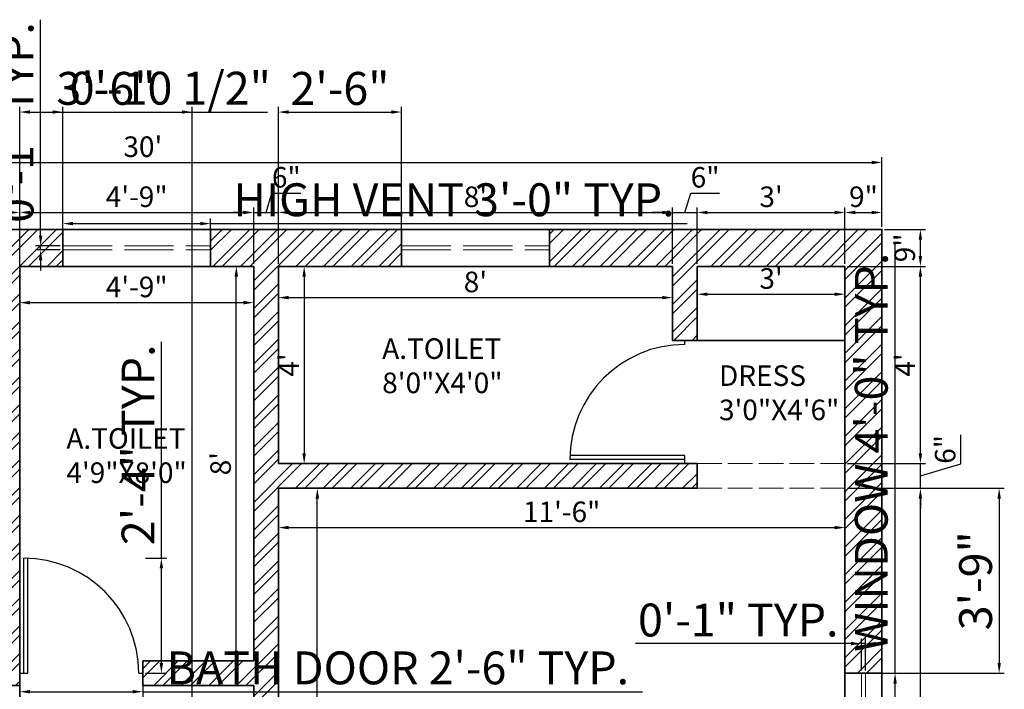
# Model space of a CAD drawing. Units: inches. Extents: x 3595 to 4516, y 2363 to 2965.
# Tile 5 of 12: x 3790 to 4030, y 2791 to 2954. Entities that reach past the tile are written whole.
import ezdxf

# ---------------------------------------------------------------- set-up
doc = ezdxf.new("R2010")
doc.units = ezdxf.units.IN
doc.linetypes.add('ACAD_ISO02W100', pattern=[15, 12, -3])
for name, color, linetype, lineweight in [('A-ANNO-DIMS', 2, 'Continuous', 18), ('A-AREA-IDEN', 7, 'Continuous', 18), ('A-DOOR', 4, 'Continuous', 25), ('A-GLAZ', 4, 'Continuous', 18), ('A-GLAZ-HIGH', 4, 'ACAD_ISO02W100', 18), ('A-WALL', 7, 'Continuous', 35), ('A-WALL-OVHD', 7, 'ACAD_ISO02W100', 18)]:
    doc.layers.add(name, color=color, linetype=linetype, lineweight=lineweight)
doc.layers.add('A-WALL-PATT', color=251, linetype='Continuous', lineweight=13, true_color=0x636466)
doc.styles.get("Standard").update_dxf_attribs({"font": 'arial.ttf'})
doc.dimstyles.new('ISO-25', dxfattribs={"dimtxt": 8, "dimasz": 2.5, "dimexe": 1.25, "dimexo": 0.625, "dimtad": 1, "dimdec": 1, "dimlunit": 3, "dimtxsty": 'Standard', "dimcen": 2.5, "dimadec": 0, "dimazin": 0, "dimtfac": 1, "dimtdec": 1, "dimtmove": 0, "dimatfit": 3, "dimfxl": 1, "dimarcsym": 0})

# ---------------------------------------------------------------- blocks, each defined once
blk = doc.blocks.new('D2')
for p, q in [((1, 0), (1, 28)), ((2, 0), (2, 27.98)), ((0, 0), (2, 0)), ((29, 0), (30, 0))]:
    blk.add_line(p, q)
at = {"ltscale": 0.5}
blk.add_arc((1, 0), 28, 0, 90, dxfattribs=at)
blk = doc.blocks.new('*D39')
at = {"layer": 'A-ANNO-DIMS', "color": 0, "lineweight": -2, "transparency": 16777216}
for p, q in [((3853.52, 2840.04), (3863.63, 2840.04)), ((3862.38, 2704.54), (3862.38, 2837.54)), ((3853.52, 2702.04), (3863.63, 2702.04))]:
    blk.add_line(p, q, dxfattribs=at)
at = {"layer": 'A-ANNO-DIMS', "color": 0, "transparency": 16777216}
for points in [[(3861.96, 2837.54), (3862.79, 2837.54), (3862.38, 2840.04)], [(3861.96, 2704.54), (3862.79, 2704.54), (3862.38, 2702.04)]]:
    blk.add_solid(points, dxfattribs=at)
at = {"layer": 'Defpoints', "color": 0, "transparency": 16777216}
for p in [(3852.89, 2840.04), (3862.38, 2840.04), (3852.89, 2702.04)]:
    blk.add_point(p, dxfattribs=at)
at = {"layer": 'A-ANNO-DIMS', "color": 0, "transparency": 16777216, "insert": (3859.2, 2771.04), "char_height": 5, "attachment_point": 5, "rotation": 90}
blk.add_mtext('11\'-6"', dxfattribs=at)
blk = doc.blocks.new('*D40')
at = {"layer": 'A-ANNO-DIMS', "color": 0, "lineweight": -2, "transparency": 16777216}
for p, q in [((3852.89, 2839.42), (3852.89, 2829.23)), ((3990.89, 2839.42), (3990.89, 2829.23)), ((3855.39, 2830.48), (3988.39, 2830.48))]:
    blk.add_line(p, q, dxfattribs=at)
at = {"layer": 'A-ANNO-DIMS', "color": 0, "transparency": 16777216}
for points in [[(3855.39, 2830.9), (3855.39, 2830.06), (3852.89, 2830.48)], [(3988.39, 2830.9), (3988.39, 2830.06), (3990.89, 2830.48)]]:
    blk.add_solid(points, dxfattribs=at)
at = {"layer": 'Defpoints', "color": 0, "transparency": 16777216}
for p in [(3852.89, 2840.04), (3990.89, 2840.04), (3990.89, 2830.48)]:
    blk.add_point(p, dxfattribs=at)
at = {"layer": 'A-ANNO-DIMS', "color": 0, "transparency": 16777216, "insert": (3921.89, 2833.66), "char_height": 5, "attachment_point": 5}
blk.add_mtext('11\'-6"', dxfattribs=at)
blk = doc.blocks.new('*D41')
at = {"layer": 'A-ANNO-DIMS', "color": 0, "lineweight": -2, "transparency": 16777216}
for p, q in [((3852.89, 2893.42), (3852.89, 2885.19)), ((3948.89, 2893.42), (3948.89, 2885.19)), ((3855.39, 2886.44), (3946.39, 2886.44))]:
    blk.add_line(p, q, dxfattribs=at)
at = {"layer": 'A-ANNO-DIMS', "color": 0, "transparency": 16777216}
for points in [[(3855.39, 2886.85), (3855.39, 2886.02), (3852.89, 2886.44)], [(3946.39, 2886.85), (3946.39, 2886.02), (3948.89, 2886.44)]]:
    blk.add_solid(points, dxfattribs=at)
at = {"layer": 'Defpoints', "color": 0, "transparency": 16777216}
for p in [(3852.89, 2894.04), (3948.89, 2894.04), (3948.89, 2886.44)]:
    blk.add_point(p, dxfattribs=at)
at = {"layer": 'A-ANNO-DIMS', "color": 0, "transparency": 16777216, "insert": (3900.89, 2889.61), "char_height": 5, "attachment_point": 5}
blk.add_mtext("8'", dxfattribs=at)
blk = doc.blocks.new('*D42')
at = {"layer": 'A-ANNO-DIMS', "color": 0, "lineweight": -2, "transparency": 16777216}
for p, q in [((3853.52, 2894.04), (3860.42, 2894.04)), ((3859.17, 2891.54), (3859.17, 2848.54)), ((3853.52, 2846.04), (3860.42, 2846.04))]:
    blk.add_line(p, q, dxfattribs=at)
at = {"layer": 'A-ANNO-DIMS', "color": 0, "transparency": 16777216}
for points in [[(3858.76, 2891.54), (3859.59, 2891.54), (3859.17, 2894.04)], [(3858.76, 2848.54), (3859.59, 2848.54), (3859.17, 2846.04)]]:
    blk.add_solid(points, dxfattribs=at)
at = {"layer": 'Defpoints', "color": 0, "transparency": 16777216}
for p in [(3852.89, 2894.04), (3852.89, 2846.04), (3859.17, 2846.04)]:
    blk.add_point(p, dxfattribs=at)
at = {"layer": 'A-ANNO-DIMS', "color": 0, "transparency": 16777216, "insert": (3856.05, 2870.04), "char_height": 5, "attachment_point": 5, "rotation": 90}
blk.add_mtext("4'", dxfattribs=at)
blk = doc.blocks.new('*D43')
at = {"layer": 'A-ANNO-DIMS', "color": 0, "lineweight": -2, "transparency": 16777216}
for p, q in [((3954.89, 2893.42), (3954.89, 2886.01)), ((3990.89, 2893.42), (3990.89, 2886.01)), ((3957.39, 2887.26), (3988.39, 2887.26))]:
    blk.add_line(p, q, dxfattribs=at)
at = {"layer": 'A-ANNO-DIMS', "color": 0, "transparency": 16777216}
for points in [[(3957.39, 2887.67), (3957.39, 2886.84), (3954.89, 2887.26)], [(3988.39, 2887.67), (3988.39, 2886.84), (3990.89, 2887.26)]]:
    blk.add_solid(points, dxfattribs=at)
at = {"layer": 'Defpoints', "color": 0, "transparency": 16777216}
for p in [(3954.89, 2894.04), (3990.89, 2894.04), (3990.89, 2887.26)]:
    blk.add_point(p, dxfattribs=at)
at = {"layer": 'A-ANNO-DIMS', "color": 0, "transparency": 16777216, "insert": (3972.89, 2890.44), "char_height": 5, "attachment_point": 5}
blk.add_mtext("3'", dxfattribs=at)
blk = doc.blocks.new('*D44')
at = {"layer": 'A-ANNO-DIMS', "color": 0, "lineweight": -2, "transparency": 16777216}
for p, q in [((3789.89, 2893.42), (3789.89, 2883.96)), ((3846.89, 2893.42), (3846.89, 2883.96)), ((3792.39, 2885.21), (3844.39, 2885.21))]:
    blk.add_line(p, q, dxfattribs=at)
at = {"layer": 'A-ANNO-DIMS', "color": 0, "transparency": 16777216}
for points in [[(3792.39, 2885.63), (3792.39, 2884.79), (3789.89, 2885.21)], [(3844.39, 2885.63), (3844.39, 2884.79), (3846.89, 2885.21)]]:
    blk.add_solid(points, dxfattribs=at)
at = {"layer": 'Defpoints', "color": 0, "transparency": 16777216}
for p in [(3789.89, 2894.04), (3846.89, 2894.04), (3846.89, 2885.21)]:
    blk.add_point(p, dxfattribs=at)
at = {"layer": 'A-ANNO-DIMS', "color": 0, "transparency": 16777216, "insert": (3818.39, 2888.39), "char_height": 5, "attachment_point": 5}
blk.add_mtext('4\'-9"', dxfattribs=at)
blk = doc.blocks.new('*D45')
at = {"layer": 'A-ANNO-DIMS', "color": 0, "lineweight": -2, "transparency": 16777216}
for p, q in [((3846.27, 2894.04), (3841.4, 2894.04)), ((3842.65, 2800.54), (3842.65, 2891.54)), ((3846.27, 2798.04), (3841.4, 2798.04))]:
    blk.add_line(p, q, dxfattribs=at)
at = {"layer": 'A-ANNO-DIMS', "color": 0, "transparency": 16777216}
for points in [[(3842.23, 2891.54), (3843.07, 2891.54), (3842.65, 2894.04)], [(3842.23, 2800.54), (3843.07, 2800.54), (3842.65, 2798.04)]]:
    blk.add_solid(points, dxfattribs=at)
at = {"layer": 'Defpoints', "color": 0, "transparency": 16777216}
for p in [(3842.65, 2894.04), (3846.89, 2894.04), (3846.89, 2798.04)]:
    blk.add_point(p, dxfattribs=at)
at = {"layer": 'A-ANNO-DIMS', "color": 0, "transparency": 16777216, "insert": (3839.47, 2846.04), "char_height": 5, "attachment_point": 5, "rotation": 90}
blk.add_mtext("8'", dxfattribs=at)
blk = doc.blocks.new('*D62')
at = {"layer": 'A-ANNO-DIMS', "color": 0, "lineweight": -2, "transparency": 16777216}
for p, q in [((3780.89, 2894.67), (3780.89, 2908.4)), ((3783.39, 2907.15), (3787.39, 2907.15)), ((3789.89, 2894.67), (3789.89, 2908.4))]:
    blk.add_line(p, q, dxfattribs=at)
at = {"layer": 'A-ANNO-DIMS', "color": 0, "transparency": 16777216}
for points in [[(3783.39, 2907.57), (3783.39, 2906.73), (3780.89, 2907.15)], [(3787.39, 2907.57), (3787.39, 2906.73), (3789.89, 2907.15)]]:
    blk.add_solid(points, dxfattribs=at)
at = {"layer": 'Defpoints', "color": 0, "transparency": 16777216}
for p in [(3789.89, 2907.15), (3780.89, 2894.04), (3789.89, 2894.04)]:
    blk.add_point(p, dxfattribs=at)
at = {"layer": 'A-ANNO-DIMS', "color": 0, "transparency": 16777216, "insert": (3785.39, 2910.33), "char_height": 5, "attachment_point": 5}
blk.add_mtext('9"', dxfattribs=at)
blk = doc.blocks.new('*D63')
at = {"layer": 'A-ANNO-DIMS', "color": 0, "lineweight": -2, "transparency": 16777216}
for p, q in [((3789.89, 2894.67), (3789.89, 2908.4)), ((3792.39, 2907.15), (3844.39, 2907.15)), ((3846.89, 2894.67), (3846.89, 2908.4))]:
    blk.add_line(p, q, dxfattribs=at)
at = {"layer": 'A-ANNO-DIMS', "color": 0, "transparency": 16777216}
for points in [[(3792.39, 2907.57), (3792.39, 2906.73), (3789.89, 2907.15)], [(3844.39, 2907.57), (3844.39, 2906.73), (3846.89, 2907.15)]]:
    blk.add_solid(points, dxfattribs=at)
at = {"layer": 'Defpoints', "color": 0, "transparency": 16777216}
for p in [(3846.89, 2907.15), (3789.89, 2894.04), (3846.89, 2894.04)]:
    blk.add_point(p, dxfattribs=at)
at = {"layer": 'A-ANNO-DIMS', "color": 0, "transparency": 16777216, "insert": (3818.39, 2910.33), "char_height": 5, "attachment_point": 5}
blk.add_mtext('4\'-9"', dxfattribs=at)
blk = doc.blocks.new('*D64')
at = {"layer": 'A-ANNO-DIMS', "color": 0, "lineweight": -2, "transparency": 16777216}
for p, q in [((3849.89, 2907.15), (3851.32, 2911.89)), ((3851.32, 2911.89), (3858.34, 2911.89)), ((3844.39, 2907.15), (3841.89, 2907.15)), ((3846.89, 2894.67), (3846.89, 2908.4)), ((3846.89, 2907.15), (3852.89, 2907.15)), ((3846.89, 2907.15), (3852.89, 2907.15)), ((3852.89, 2894.67), (3852.89, 2908.4)), ((3855.39, 2907.15), (3857.89, 2907.15))]:
    blk.add_line(p, q, dxfattribs=at)
at = {"layer": 'A-ANNO-DIMS', "color": 0, "transparency": 16777216}
for points in [[(3844.39, 2907.57), (3844.39, 2906.73), (3846.89, 2907.15)], [(3855.39, 2907.57), (3855.39, 2906.73), (3852.89, 2907.15)]]:
    blk.add_solid(points, dxfattribs=at)
at = {"layer": 'Defpoints', "color": 0, "transparency": 16777216}
for p in [(3852.89, 2907.15), (3846.89, 2894.04), (3852.89, 2894.04)]:
    blk.add_point(p, dxfattribs=at)
at = {"layer": 'A-ANNO-DIMS', "color": 0, "transparency": 16777216, "insert": (3854.83, 2915.07), "char_height": 5, "attachment_point": 5}
blk.add_mtext('6"', dxfattribs=at)
blk = doc.blocks.new('*D65')
at = {"layer": 'A-ANNO-DIMS', "color": 0, "lineweight": -2, "transparency": 16777216}
for p, q in [((3852.89, 2894.67), (3852.89, 2908.4)), ((3855.39, 2907.15), (3946.39, 2907.15)), ((3948.89, 2894.67), (3948.89, 2908.4))]:
    blk.add_line(p, q, dxfattribs=at)
at = {"layer": 'A-ANNO-DIMS', "color": 0, "transparency": 16777216}
for points in [[(3855.39, 2907.57), (3855.39, 2906.73), (3852.89, 2907.15)], [(3946.39, 2907.57), (3946.39, 2906.73), (3948.89, 2907.15)]]:
    blk.add_solid(points, dxfattribs=at)
at = {"layer": 'Defpoints', "color": 0, "transparency": 16777216}
for p in [(3948.89, 2907.15), (3852.89, 2894.04), (3948.89, 2894.04)]:
    blk.add_point(p, dxfattribs=at)
at = {"layer": 'A-ANNO-DIMS', "color": 0, "transparency": 16777216, "insert": (3900.89, 2910.33), "char_height": 5, "attachment_point": 5}
blk.add_mtext("8'", dxfattribs=at)
blk = doc.blocks.new('*D66')
at = {"layer": 'A-ANNO-DIMS', "color": 0, "lineweight": -2, "transparency": 16777216}
for p, q in [((3951.89, 2907.15), (3953.32, 2911.89)), ((3953.32, 2911.89), (3960.34, 2911.89)), ((3946.39, 2907.15), (3943.89, 2907.15)), ((3948.89, 2894.67), (3948.89, 2908.4)), ((3948.89, 2907.15), (3954.89, 2907.15)), ((3948.89, 2907.15), (3954.89, 2907.15)), ((3954.89, 2894.67), (3954.89, 2908.4)), ((3957.39, 2907.15), (3959.89, 2907.15))]:
    blk.add_line(p, q, dxfattribs=at)
at = {"layer": 'A-ANNO-DIMS', "color": 0, "transparency": 16777216}
for points in [[(3946.39, 2907.57), (3946.39, 2906.73), (3948.89, 2907.15)], [(3957.39, 2907.57), (3957.39, 2906.73), (3954.89, 2907.15)]]:
    blk.add_solid(points, dxfattribs=at)
at = {"layer": 'Defpoints', "color": 0, "transparency": 16777216}
for p in [(3954.89, 2907.15), (3948.89, 2894.04), (3954.89, 2894.04)]:
    blk.add_point(p, dxfattribs=at)
at = {"layer": 'A-ANNO-DIMS', "color": 0, "transparency": 16777216, "insert": (3956.83, 2915.07), "char_height": 5, "attachment_point": 5}
blk.add_mtext('6"', dxfattribs=at)
blk = doc.blocks.new('*D67')
at = {"layer": 'A-ANNO-DIMS', "color": 0, "lineweight": -2, "transparency": 16777216}
for p, q in [((3954.89, 2894.67), (3954.89, 2908.4)), ((3957.39, 2907.15), (3988.39, 2907.15)), ((3990.89, 2894.67), (3990.89, 2908.4))]:
    blk.add_line(p, q, dxfattribs=at)
at = {"layer": 'A-ANNO-DIMS', "color": 0, "transparency": 16777216}
for points in [[(3957.39, 2907.57), (3957.39, 2906.73), (3954.89, 2907.15)], [(3988.39, 2907.57), (3988.39, 2906.73), (3990.89, 2907.15)]]:
    blk.add_solid(points, dxfattribs=at)
at = {"layer": 'Defpoints', "color": 0, "transparency": 16777216}
for p in [(3990.89, 2907.15), (3954.89, 2894.04), (3990.89, 2894.04)]:
    blk.add_point(p, dxfattribs=at)
at = {"layer": 'A-ANNO-DIMS', "color": 0, "transparency": 16777216, "insert": (3972.89, 2910.33), "char_height": 5, "attachment_point": 5}
blk.add_mtext("3'", dxfattribs=at)
blk = doc.blocks.new('*D68')
at = {"layer": 'A-ANNO-DIMS', "color": 0, "lineweight": -2, "transparency": 16777216}
for p, q in [((3990.89, 2894.67), (3990.89, 2908.4)), ((3993.39, 2907.15), (3997.39, 2907.15)), ((3999.89, 2903.67), (3999.89, 2908.4))]:
    blk.add_line(p, q, dxfattribs=at)
at = {"layer": 'A-ANNO-DIMS', "color": 0, "transparency": 16777216}
for points in [[(3993.39, 2907.57), (3993.39, 2906.73), (3990.89, 2907.15)], [(3997.39, 2907.57), (3997.39, 2906.73), (3999.89, 2907.15)]]:
    blk.add_solid(points, dxfattribs=at)
at = {"layer": 'Defpoints', "color": 0, "transparency": 16777216}
for p in [(3999.89, 2907.15), (3999.89, 2903.04), (3990.89, 2894.04)]:
    blk.add_point(p, dxfattribs=at)
at = {"layer": 'A-ANNO-DIMS', "color": 0, "transparency": 16777216, "insert": (3995.39, 2910.33), "char_height": 5, "attachment_point": 5}
blk.add_mtext('9"', dxfattribs=at)
blk = doc.blocks.new('*D85')
at = {"layer": 'A-ANNO-DIMS', "color": 0, "lineweight": -2, "transparency": 16777216}
for p, q in [((3991.52, 2840.04), (4010.51, 2840.04)), ((4009.26, 2704.54), (4009.26, 2837.54)), ((3991.52, 2702.04), (4010.51, 2702.04))]:
    blk.add_line(p, q, dxfattribs=at)
at = {"layer": 'A-ANNO-DIMS', "color": 0, "transparency": 16777216}
for points in [[(4008.84, 2837.54), (4009.67, 2837.54), (4009.26, 2840.04)], [(4008.84, 2704.54), (4009.67, 2704.54), (4009.26, 2702.04)]]:
    blk.add_solid(points, dxfattribs=at)
at = {"layer": 'Defpoints', "color": 0, "transparency": 16777216}
for p in [(3990.89, 2840.04), (4009.26, 2840.04), (3990.89, 2702.04)]:
    blk.add_point(p, dxfattribs=at)
at = {"layer": 'A-ANNO-DIMS', "color": 0, "transparency": 16777216, "insert": (4006.08, 2771.04), "char_height": 5, "attachment_point": 5, "rotation": 90}
blk.add_mtext('11\'-6"', dxfattribs=at)
blk = doc.blocks.new('*D86')
at = {"layer": 'A-ANNO-DIMS', "color": 0, "lineweight": -2, "transparency": 16777216}
for p, q in [((4019.1, 2846), (4019.1, 2853.02)), ((4009.26, 2848.54), (4009.26, 2851.04)), ((3991.52, 2846.04), (4010.51, 2846.04)), ((4009.26, 2840.04), (4009.26, 2846.04)), ((4009.26, 2840.04), (4009.26, 2846.04)), ((4009.26, 2843.04), (4019.1, 2846)), ((3991.52, 2840.04), (4010.51, 2840.04)), ((4009.26, 2837.54), (4009.26, 2835.04))]:
    blk.add_line(p, q, dxfattribs=at)
at = {"layer": 'A-ANNO-DIMS', "color": 0, "transparency": 16777216}
for points in [[(4008.84, 2848.54), (4009.67, 2848.54), (4009.26, 2846.04)], [(4008.84, 2837.54), (4009.67, 2837.54), (4009.26, 2840.04)]]:
    blk.add_solid(points, dxfattribs=at)
at = {"layer": 'Defpoints', "color": 0, "transparency": 16777216}
for p in [(3990.89, 2846.04), (4009.26, 2846.04), (3990.89, 2840.04)]:
    blk.add_point(p, dxfattribs=at)
at = {"layer": 'A-ANNO-DIMS', "color": 0, "transparency": 16777216, "insert": (4015.93, 2849.51), "char_height": 5, "attachment_point": 5, "rotation": 90}
blk.add_mtext('6"', dxfattribs=at)
blk = doc.blocks.new('*D87')
at = {"layer": 'A-ANNO-DIMS', "color": 0, "lineweight": -2, "transparency": 16777216}
for p, q in [((3991.52, 2894.04), (4010.51, 2894.04)), ((4009.26, 2848.54), (4009.26, 2891.54)), ((3991.52, 2846.04), (4010.51, 2846.04))]:
    blk.add_line(p, q, dxfattribs=at)
at = {"layer": 'A-ANNO-DIMS', "color": 0, "transparency": 16777216}
for points in [[(4008.84, 2891.54), (4009.67, 2891.54), (4009.26, 2894.04)], [(4008.84, 2848.54), (4009.67, 2848.54), (4009.26, 2846.04)]]:
    blk.add_solid(points, dxfattribs=at)
at = {"layer": 'Defpoints', "color": 0, "transparency": 16777216}
for p in [(3990.89, 2894.04), (4009.26, 2894.04), (3990.89, 2846.04)]:
    blk.add_point(p, dxfattribs=at)
at = {"layer": 'A-ANNO-DIMS', "color": 0, "transparency": 16777216, "insert": (4006.13, 2870.04), "char_height": 5, "attachment_point": 5, "rotation": 90}
blk.add_mtext("4'", dxfattribs=at)
blk = doc.blocks.new('*D88')
at = {"layer": 'A-ANNO-DIMS', "color": 0, "lineweight": -2, "transparency": 16777216}
for p, q in [((4000.52, 2903.04), (4010.51, 2903.04)), ((4009.26, 2896.54), (4009.26, 2900.54)), ((3991.52, 2894.04), (4010.51, 2894.04))]:
    blk.add_line(p, q, dxfattribs=at)
at = {"layer": 'A-ANNO-DIMS', "color": 0, "transparency": 16777216}
for points in [[(4008.84, 2900.54), (4009.67, 2900.54), (4009.26, 2903.04)], [(4008.84, 2896.54), (4009.67, 2896.54), (4009.26, 2894.04)]]:
    blk.add_solid(points, dxfattribs=at)
at = {"layer": 'Defpoints', "color": 0, "transparency": 16777216}
for p in [(3999.89, 2903.04), (4009.26, 2903.04), (3990.89, 2894.04)]:
    blk.add_point(p, dxfattribs=at)
at = {"layer": 'A-ANNO-DIMS', "color": 0, "transparency": 16777216, "insert": (4006.08, 2898.54), "char_height": 5, "attachment_point": 5, "rotation": 90}
blk.add_mtext('9"', dxfattribs=at)
blk = doc.blocks.new('*D89')
at = {"layer": 'A-ANNO-DIMS', "color": 0, "lineweight": -2, "transparency": 16777216}
for p, q in [((3639.89, 2903.67), (3639.89, 2920.58)), ((3642.39, 2919.33), (3997.39, 2919.33)), ((3999.89, 2903.67), (3999.89, 2920.58))]:
    blk.add_line(p, q, dxfattribs=at)
at = {"layer": 'A-ANNO-DIMS', "color": 0, "transparency": 16777216}
for points in [[(3642.39, 2919.75), (3642.39, 2918.91), (3639.89, 2919.33)], [(3997.39, 2919.75), (3997.39, 2918.91), (3999.89, 2919.33)]]:
    blk.add_solid(points, dxfattribs=at)
at = {"layer": 'Defpoints', "color": 0, "transparency": 16777216}
for p in [(3999.89, 2919.33), (3639.89, 2903.04), (3999.89, 2903.04)]:
    blk.add_point(p, dxfattribs=at)
at = {"layer": 'A-ANNO-DIMS', "color": 0, "transparency": 16777216, "insert": (3819.89, 2922.51), "char_height": 5, "attachment_point": 5}
blk.add_mtext("30'", dxfattribs=at)
blk = doc.blocks.new('VENT-GLAZING-36IN')
for p, q in [((0, 1), (36, 1)), ((0, 0), (36, 0))]:
    blk.add_line(p, q)
blk = doc.blocks.new('WIN-GLAZING-48IN')
for p, q in [((0, 1), (48, 1)), ((0, 0), (48, 0))]:
    blk.add_line(p, q)
blk = doc.blocks.new('*D99')
at = {"layer": 'A-ANNO-DIMS', "color": 0, "lineweight": -2, "transparency": 16777216}
for p, q in [((4003.09, 2795.04), (4003.09, 2900.03)), ((3996.52, 2795.04), (4004.34, 2795.04)), ((4003.09, 2749.54), (4003.09, 2792.54)), ((3996.52, 2747.04), (4004.34, 2747.04))]:
    blk.add_line(p, q, dxfattribs=at)
at = {"layer": 'A-ANNO-DIMS', "color": 0, "transparency": 16777216}
for points in [[(4002.68, 2792.54), (4003.51, 2792.54), (4003.09, 2795.04)], [(4002.68, 2749.54), (4003.51, 2749.54), (4003.09, 2747.04)]]:
    blk.add_solid(points, dxfattribs=at)
at = {"layer": 'Defpoints', "color": 0, "transparency": 16777216}
for p in [(3995.89, 2795.04), (4003.09, 2795.04), (3995.89, 2747.04)]:
    blk.add_point(p, dxfattribs=at)
at = {"layer": 'A-ANNO-DIMS', "color": 0, "transparency": 16777216, "insert": (3998.33, 2848.79), "char_height": 8, "attachment_point": 5, "rotation": 90}
blk.add_mtext('WINDOW 4\'-0" TYP.', dxfattribs=at)
blk = doc.blocks.new('*D100')
at = {"layer": 'A-ANNO-DIMS', "color": 0, "lineweight": -2, "transparency": 16777216}
for p, q in [((3994.89, 2795.67), (3994.89, 2803.49)), ((3995.89, 2795.67), (3995.89, 2803.49)), ((3992.39, 2802.24), (3939.88, 2802.24)), ((3995.89, 2802.24), (3994.89, 2802.24)), ((3998.39, 2802.24), (4000.89, 2802.24))]:
    blk.add_line(p, q, dxfattribs=at)
at = {"layer": 'A-ANNO-DIMS', "color": 0, "transparency": 16777216}
for points in [[(3992.39, 2802.66), (3992.39, 2801.83), (3994.89, 2802.24)], [(3998.39, 2802.66), (3998.39, 2801.83), (3995.89, 2802.24)]]:
    blk.add_solid(points, dxfattribs=at)
at = {"layer": 'Defpoints', "color": 0, "transparency": 16777216}
for p in [(3994.89, 2802.24), (3994.89, 2795.04), (3995.89, 2795.04)]:
    blk.add_point(p, dxfattribs=at)
at = {"layer": 'A-ANNO-DIMS', "color": 0, "transparency": 16777216, "insert": (3964.89, 2806.95), "char_height": 8, "attachment_point": 5}
blk.add_mtext('0\'-1" TYP.', dxfattribs=at)
blk = doc.blocks.new('*D107')
at = {"layer": 'A-ANNO-DIMS', "color": 0, "lineweight": -2, "transparency": 16777216}
for p, q in [((3800.39, 2899.67), (3800.39, 2905.69)), ((3802.89, 2904.44), (3833.89, 2904.44)), ((3836.39, 2899.67), (3836.39, 2905.69)), ((3836.39, 2904.44), (3952.43, 2904.44))]:
    blk.add_line(p, q, dxfattribs=at)
at = {"layer": 'A-ANNO-DIMS', "color": 0, "transparency": 16777216}
for points in [[(3802.89, 2904.86), (3802.89, 2904.03), (3800.39, 2904.44)], [(3833.89, 2904.86), (3833.89, 2904.03), (3836.39, 2904.44)]]:
    blk.add_solid(points, dxfattribs=at)
at = {"layer": 'Defpoints', "color": 0, "transparency": 16777216}
for p in [(3836.39, 2904.44), (3800.39, 2899.04), (3836.39, 2899.04)]:
    blk.add_point(p, dxfattribs=at)
at = {"layer": 'A-ANNO-DIMS', "color": 0, "transparency": 16777216, "insert": (3895.66, 2909.21), "char_height": 8, "attachment_point": 5}
blk.add_mtext('HIGH VENT 3\'-0" TYP.', dxfattribs=at)
blk = doc.blocks.new('*D108')
at = {"layer": 'A-ANNO-DIMS', "color": 0, "lineweight": -2, "transparency": 16777216}
for p, q in [((3794.99, 2901.54), (3794.99, 2954.06)), ((3799.77, 2899.04), (3793.74, 2899.04)), ((3799.77, 2898.04), (3793.74, 2898.04)), ((3794.99, 2898.04), (3794.99, 2899.04)), ((3794.99, 2895.54), (3794.99, 2893.04))]:
    blk.add_line(p, q, dxfattribs=at)
at = {"layer": 'A-ANNO-DIMS', "color": 0, "transparency": 16777216}
for points in [[(3794.58, 2901.54), (3795.41, 2901.54), (3794.99, 2899.04)], [(3794.58, 2895.54), (3795.41, 2895.54), (3794.99, 2898.04)]]:
    blk.add_solid(points, dxfattribs=at)
at = {"layer": 'Defpoints', "color": 0, "transparency": 16777216}
for p in [(3794.99, 2899.04), (3800.39, 2899.04), (3800.39, 2898.04)]:
    blk.add_point(p, dxfattribs=at)
at = {"layer": 'A-ANNO-DIMS', "color": 0, "transparency": 16777216, "insert": (3790.28, 2929.05), "char_height": 8, "attachment_point": 5, "rotation": 90}
blk.add_mtext('0\'-1" TYP.', dxfattribs=at)
blk = doc.blocks.new('*D109')
at = {"layer": 'A-ANNO-DIMS', "color": 0, "lineweight": -2, "transparency": 16777216}
for p, q in [((3789.89, 2794.42), (3789.89, 2789.29)), ((3819.89, 2794.42), (3819.89, 2789.29)), ((3792.39, 2790.54), (3817.39, 2790.54)), ((3819.89, 2790.54), (3941.6, 2790.54))]:
    blk.add_line(p, q, dxfattribs=at)
at = {"layer": 'A-ANNO-DIMS', "color": 0, "transparency": 16777216}
for points in [[(3792.39, 2790.96), (3792.39, 2790.13), (3789.89, 2790.54)], [(3817.39, 2790.96), (3817.39, 2790.13), (3819.89, 2790.54)]]:
    blk.add_solid(points, dxfattribs=at)
at = {"layer": 'Defpoints', "color": 0, "transparency": 16777216}
for p in [(3789.89, 2795.04), (3819.89, 2795.04), (3819.89, 2790.54)]:
    blk.add_point(p, dxfattribs=at)
at = {"layer": 'A-ANNO-DIMS', "color": 0, "transparency": 16777216, "insert": (3881.99, 2795.31), "char_height": 8, "attachment_point": 5}
blk.add_mtext('BATH DOOR 2\'-6" TYP.', dxfattribs=at)
blk = doc.blocks.new('*D110')
at = {"layer": 'A-ANNO-DIMS', "color": 0, "lineweight": -2, "transparency": 16777216}
for p, q in [((3824.39, 2823.04), (3824.39, 2875.69)), ((3820.52, 2823.04), (3825.64, 2823.04)), ((3824.39, 2797.54), (3824.39, 2820.54)), ((3820.52, 2795.04), (3825.64, 2795.04))]:
    blk.add_line(p, q, dxfattribs=at)
at = {"layer": 'A-ANNO-DIMS', "color": 0, "transparency": 16777216}
for points in [[(3823.98, 2820.54), (3824.81, 2820.54), (3824.39, 2823.04)], [(3823.98, 2797.54), (3824.81, 2797.54), (3824.39, 2795.04)]]:
    blk.add_solid(points, dxfattribs=at)
at = {"layer": 'Defpoints', "color": 0, "transparency": 16777216}
for p in [(3819.89, 2823.04), (3824.39, 2823.04), (3819.89, 2795.04)]:
    blk.add_point(p, dxfattribs=at)
at = {"layer": 'A-ANNO-DIMS', "color": 0, "transparency": 16777216, "insert": (3819.75, 2850.62), "char_height": 8, "attachment_point": 5, "rotation": 90}
blk.add_mtext('2\'-4" TYP.', dxfattribs=at)
blk = doc.blocks.new('*D148')
at = {"layer": 'A-ANNO-DIMS', "color": 0, "lineweight": -2, "transparency": 16777216}
for p, q in [((3789.89, 2894.67), (3789.89, 2932.84)), ((3800.39, 2894.67), (3800.39, 2932.84)), ((3792.39, 2931.59), (3797.89, 2931.59)), ((3800.39, 2931.59), (3850.27, 2931.59))]:
    blk.add_line(p, q, dxfattribs=at)
at = {"layer": 'A-ANNO-DIMS', "color": 0, "transparency": 16777216}
for points in [[(3792.39, 2932.01), (3792.39, 2931.18), (3789.89, 2931.59)], [(3797.89, 2932.01), (3797.89, 2931.18), (3800.39, 2931.59)]]:
    blk.add_solid(points, dxfattribs=at)
at = {"layer": 'Defpoints', "color": 0, "transparency": 16777216}
for p in [(3800.39, 2931.59), (3789.89, 2894.04), (3800.39, 2894.04)]:
    blk.add_point(p, dxfattribs=at)
at = {"layer": 'A-ANNO-DIMS', "color": 0, "transparency": 16777216, "insert": (3826.58, 2936.36), "char_height": 8, "attachment_point": 5}
blk.add_mtext('0\'-10 1/2"', dxfattribs=at)
blk = doc.blocks.new('*D149')
at = {"layer": 'A-ANNO-DIMS', "color": 0, "lineweight": -2, "transparency": 16777216}
for p, q in [((3852.89, 2894.67), (3852.89, 2932.84)), ((3882.89, 2894.67), (3882.89, 2932.84)), ((3855.39, 2931.59), (3880.39, 2931.59))]:
    blk.add_line(p, q, dxfattribs=at)
at = {"layer": 'A-ANNO-DIMS', "color": 0, "transparency": 16777216}
for points in [[(3855.39, 2932.01), (3855.39, 2931.18), (3852.89, 2931.59)], [(3880.39, 2932.01), (3880.39, 2931.18), (3882.89, 2931.59)]]:
    blk.add_solid(points, dxfattribs=at)
at = {"layer": 'Defpoints', "color": 0, "transparency": 16777216}
for p in [(3882.89, 2931.59), (3852.89, 2894.04), (3882.89, 2894.04)]:
    blk.add_point(p, dxfattribs=at)
at = {"layer": 'A-ANNO-DIMS', "color": 0, "transparency": 16777216, "insert": (3867.89, 2936.3), "char_height": 8, "attachment_point": 5}
blk.add_mtext('2\'-6"', dxfattribs=at)
blk = doc.blocks.new('*D153')
at = {"layer": 'A-ANNO-DIMS', "color": 0, "lineweight": -2, "transparency": 16777216}
for p, q in [((3991.52, 2840.04), (4029.69, 2840.04)), ((4028.44, 2837.54), (4028.44, 2797.54)), ((3991.52, 2795.04), (4029.69, 2795.04))]:
    blk.add_line(p, q, dxfattribs=at)
at = {"layer": 'A-ANNO-DIMS', "color": 0, "transparency": 16777216}
for points in [[(4028.03, 2837.54), (4028.86, 2837.54), (4028.44, 2840.04)], [(4028.03, 2797.54), (4028.86, 2797.54), (4028.44, 2795.04)]]:
    blk.add_solid(points, dxfattribs=at)
at = {"layer": 'Defpoints', "color": 0, "transparency": 16777216}
for p in [(3990.89, 2840.04), (3990.89, 2795.04), (4028.44, 2795.04)]:
    blk.add_point(p, dxfattribs=at)
at = {"layer": 'A-ANNO-DIMS', "color": 0, "transparency": 16777216, "insert": (4023.73, 2817.54), "char_height": 8, "attachment_point": 5, "rotation": 90}
blk.add_mtext('3\'-9"', dxfattribs=at)
blk = doc.blocks.new('*D157')
at = {"layer": 'A-ANNO-DIMS', "color": 0, "lineweight": -2, "transparency": 16777216}
for p, q in [((3789.89, 2486.67), (3789.89, 2932.84)), ((3831.89, 2486.67), (3831.89, 2932.84)), ((3792.39, 2931.59), (3829.39, 2931.59))]:
    blk.add_line(p, q, dxfattribs=at)
at = {"layer": 'A-ANNO-DIMS', "color": 0, "transparency": 16777216}
for points in [[(3792.39, 2932.01), (3792.39, 2931.18), (3789.89, 2931.59)], [(3829.39, 2932.01), (3829.39, 2931.18), (3831.89, 2931.59)]]:
    blk.add_solid(points, dxfattribs=at)
at = {"layer": 'Defpoints', "color": 0, "transparency": 16777216}
for p in [(3831.89, 2931.59), (3789.89, 2486.04), (3831.89, 2486.04)]:
    blk.add_point(p, dxfattribs=at)
at = {"layer": 'A-ANNO-DIMS', "color": 0, "transparency": 16777216, "insert": (3810.89, 2936.31), "char_height": 8, "attachment_point": 5}
blk.add_mtext('3\'-6"', dxfattribs=at)

msp = doc.modelspace()

# ---------------------------------------------------------------- hatches: boundary and pattern name
at = {"layer": 'A-WALL-PATT'}
h = msp.add_hatch(dxfattribs=at)
h.set_pattern_fill('ANSI32', color=256, scale=0.5)
h.paths.add_polyline_path([(3648.89, 2894.04), (3726.89, 2894.04), (3726.89, 2903.04), (3639.89, 2903.04), (3639.89, 2756.04), (3648.89, 2756.04)])
h.paths.add_polyline_path([(3800.39, 2903.04), (3774.89, 2903.04), (3774.89, 2894.04), (3780.89, 2894.04), (3780.89, 2792.04), (3789.89, 2792.04), (3789.89, 2894.04), (3800.39, 2894.04)])
h.paths.add_polyline_path([(3882.89, 2903.04), (3836.39, 2903.04), (3836.39, 2894.04), (3846.89, 2894.04), (3846.89, 2798.04), (3819.89, 2798.04), (3819.89, 2792.04), (3846.89, 2792.04), (3846.89, 2756.04), (3780.89, 2756.04), (3780.89, 2702.04), (3777.89, 2702.04), (3777.89, 2693.04), (3800.39, 2693.04), (3800.39, 2702.04), (3789.89, 2702.04), (3789.89, 2750.04), (3846.89, 2750.04), (3846.89, 2702.04), (3836.39, 2702.04), (3836.39, 2693.04), (3951.89, 2693.04), (3951.89, 2702.04), (3852.89, 2702.04), (3852.89, 2840.04), (3954.89, 2840.04), (3954.89, 2846.04), (3852.89, 2846.04), (3852.89, 2894.04), (3882.89, 2894.04)])
h.paths.add_polyline_path([(3999.89, 2903.04), (3918.89, 2903.04), (3918.89, 2894.04), (3948.89, 2894.04), (3948.89, 2876.04), (3954.89, 2876.04), (3954.89, 2894.04), (3990.89, 2894.04), (3990.89, 2795.04), (3999.89, 2795.04)])
h.paths.add_polyline_path([(3741.89, 2702.04), (3648.89, 2702.04), (3648.89, 2708.04), (3639.89, 2708.04), (3639.89, 2673.54), (3648.89, 2673.54), (3648.89, 2693.04), (3741.89, 2693.04)])
h.paths.add_polyline_path([(3648.89, 2600.04), (3741.89, 2600.04), (3741.89, 2606.04), (3648.89, 2606.04), (3648.89, 2625.54), (3639.89, 2625.54), (3639.89, 2561.04), (3648.89, 2561.04)])
h.paths.add_polyline_path([(3648.89, 2525.04), (3639.89, 2525.04), (3639.89, 2399.04), (3789.89, 2399.04), (3789.89, 2405.04), (3648.89, 2405.04), (3648.89, 2477.04), (3738.89, 2477.04), (3738.89, 2486.04), (3648.89, 2486.04)])
h.paths.add_polyline_path([(3789.89, 2606.04), (3777.89, 2606.04), (3777.89, 2600.04), (3780.89, 2600.04), (3780.89, 2486.04), (3774.89, 2486.04), (3774.89, 2477.04), (3831.89, 2477.04), (3831.89, 2486.04), (3789.89, 2486.04)])
h.paths.add_polyline_path([(3939.89, 2486.04), (3897.89, 2486.04), (3897.89, 2477.04), (3939.89, 2477.04)])
h.paths.add_polyline_path([(3999.89, 2511.54), (3990.89, 2511.54), (3990.89, 2486.04), (3987.89, 2486.04), (3987.89, 2477.04), (3999.89, 2477.04)])
h.paths.add_polyline_path([(3999.89, 2607.54), (3990.89, 2607.54), (3990.89, 2571.54), (3999.89, 2571.54)])
h.paths.add_polyline_path([(3999.89, 2747.04), (3990.89, 2747.04), (3990.89, 2702.04), (3987.89, 2702.04), (3987.89, 2693.04), (3990.89, 2693.04), (3990.89, 2667.54), (3999.89, 2667.54)])

# ---------------------------------------------------------------- linework, layer by layer
at = {"layer": 'A-WALL'}
for p, q in [((3800.39, 2894.04), (3800.39, 2903.04)), ((3836.39, 2894.04), (3836.39, 2903.04)), ((3882.89, 2894.04), (3882.89, 2903.04)), ((3918.89, 2894.04), (3918.89, 2903.04)), ((3789.89, 2894.04), (3846.89, 2894.04)), ((3789.89, 2792.04), (3789.89, 2894.04)), ((3846.89, 2798.04), (3846.89, 2894.04)), ((3852.89, 2894.04), (3852.89, 2846.04)), ((3852.89, 2894.04), (3948.89, 2894.04)), ((3948.89, 2894.04), (3948.89, 2876.04)), ((3954.89, 2894.04), (3954.89, 2876.04)), ((3954.89, 2894.04), (3990.89, 2894.04)), ((3990.89, 2894.04), (3990.89, 2702.04)), ((3948.89, 2876.04), (3990.89, 2876.04)), ((3852.89, 2846.04), (3954.89, 2846.04)), ((3954.89, 2846.04), (3954.89, 2840.04)), ((3852.89, 2840.04), (3954.89, 2840.04)), ((3852.89, 2840.04), (3852.89, 2702.04)), ((3819.89, 2798.04), (3846.89, 2798.04)), ((3819.89, 2792.04), (3819.89, 2798.04)), ((3990.89, 2795.04), (3999.89, 2795.04)), ((3780.89, 2792.04), (3789.89, 2792.04)), ((3819.89, 2792.04), (3846.89, 2792.04)), ((3846.89, 2756.04), (3846.89, 2792.04))]:
    msp.add_line(p, q, dxfattribs=at)
msp.add_lwpolyline([(3789.89, 2399.04), (3639.89, 2399.04), (3639.89, 2903.04), (3999.89, 2903.04), (3999.89, 2477.04)], dxfattribs=at)
at = {"layer": 'A-WALL-OVHD', "ltscale": 0.5}
for p, q in [((3954.89, 2846.04), (3990.89, 2846.04)), ((3954.89, 2840.04), (3990.89, 2840.04))]:
    msp.add_line(p, q, dxfattribs=at)

# ---------------------------------------------------------------- block references
at = {"layer": 'A-DOOR', "rotation": 90}
msp.add_blockref('D2', (3951.89, 2846.04), dxfattribs=at)
at = {"layer": 'A-DOOR'}
msp.add_blockref('D2', (3789.89, 2795.04), dxfattribs=at)
at = {"layer": 'A-GLAZ', "rotation": 90.00000000000108}
msp.add_blockref('WIN-GLAZING-48IN', (3995.89, 2747.04), dxfattribs=at)
at = {"layer": 'A-GLAZ-HIGH'}
for p in [(3800.39, 2898.04), (3882.89, 2898.04)]:
    msp.add_blockref('VENT-GLAZING-36IN', p, dxfattribs=at)

# ---------------------------------------------------------------- texts
at = {"layer": 'A-AREA-IDEN', "char_height": 5, "attachment_point": 1}
for s, insert in [('{\\fTimes New Roman|b0|i0|c0|p18;A.TOILET\\P8\'0"X4\'0"}', (3878.18, 2876.52)), ('{\\fTimes New Roman|b0|i0|c0|p18;DRESS\\P3\'0"X4\'6"}', (3960.21, 2869.95)), ('{\\fTimes New Roman|b0|i0|c0|p18;A.TOILET\\P4\'9"X8\'0"}', (3801.27, 2854.67))]:
    msp.add_mtext_dynamic_manual_height_columns(s, width=67.3508, gutter_width=12.5, heights=[0], dxfattribs=dict(at, insert=insert))

# ---------------------------------------------------------------- dimensions: what is measured, and where the dimension line sits
at = {"layer": 'A-ANNO-DIMS'}
for base, p1, p2, angle, text, picture, middle in [((3794.99, 2899.04), (3800.39, 2898.04), (3800.39, 2899.04), 90, '<> TYP.', '*D108', (3790.28, 2929.05)), ((4003.09, 2795.04), (3995.89, 2747.04), (3995.89, 2795.04), 90, 'WINDOW <> TYP.', '*D99', (3998.33, 2848.79)), ((3824.39, 2823.04), (3819.89, 2795.04), (3819.89, 2823.04), 90, '<> TYP.', '*D110', (3819.75, 2850.62)), ((3994.89, 2802.24), (3995.89, 2795.04), (3994.89, 2795.04), 180, '<> TYP.', '*D100', (3964.89, 2806.95))]:
    dim = msp.add_linear_dim(base=base, p1=p1, p2=p2, angle=angle, text=text, dimstyle='ISO-25', override={"dimdec": 1, "dimlfac": 1, "dimrnd": 0, "dimzin": 1, "dimdsep": 46, "dimlunit": 4, "dimfrac": 2}, dxfattribs=at)
    dim.commit()
    dim.dimension.update_dxf_attribs({"geometry": picture, "text_midpoint": middle})
for base, p1, p2, override, picture, middle in [((3800.39, 2931.59), (3789.89, 2894.04), (3800.39, 2894.04), {"dimdec": 1, "dimlfac": 1, "dimrnd": 0, "dimzin": 1, "dimdsep": 46, "dimlunit": 4, "dimfrac": 2}, '*D148', (3826.58, 2936.36)), ((3831.89, 2931.59), (3789.89, 2486.04), (3831.89, 2486.04), {"dimdec": 1, "dimlfac": 1, "dimrnd": 0, "dimzin": 1, "dimdsep": 46, "dimlunit": 4, "dimfrac": 2}, '*D157', (3810.89, 2936.31)), ((3882.89, 2931.59), (3852.89, 2894.04), (3882.89, 2894.04), {"dimdec": 1, "dimlfac": 1, "dimrnd": 0, "dimzin": 1, "dimdsep": 46, "dimlunit": 4, "dimfrac": 2}, '*D149', (3867.89, 2936.3)), ((3999.89, 2919.33), (3639.89, 2903.04), (3999.89, 2903.04), {"dimtxt": 5, "dimclrd": 0, "dimclre": 0, "dimclrt": 0}, '*D89', (3819.89, 2922.51)), ((3852.89, 2907.15), (3846.89, 2894.04), (3852.89, 2894.04), {"dimtxt": 5, "dimclrd": 0, "dimclre": 0, "dimclrt": 0, "dimtmove": 1}, '*D64', (3851.94, 2915.07)), ((3954.89, 2907.15), (3948.89, 2894.04), (3954.89, 2894.04), {"dimtxt": 5, "dimclrd": 0, "dimclre": 0, "dimclrt": 0, "dimtmove": 1}, '*D66', (3953.94, 2915.07)), ((3789.89, 2907.15), (3780.89, 2894.04), (3789.89, 2894.04), {"dimtxt": 5, "dimclrd": 0, "dimclre": 0, "dimclrt": 0, "dimtmove": 1}, '*D62', (3785.39, 2910.33)), ((3846.89, 2907.15), (3789.89, 2894.04), (3846.89, 2894.04), {"dimtxt": 5, "dimclrd": 0, "dimclre": 0, "dimclrt": 0, "dimtmove": 1}, '*D63', (3818.39, 2910.33)), ((3948.89, 2907.15), (3852.89, 2894.04), (3948.89, 2894.04), {"dimtxt": 5, "dimclrd": 0, "dimclre": 0, "dimclrt": 0, "dimtmove": 1}, '*D65', (3900.89, 2910.33)), ((3990.89, 2907.15), (3954.89, 2894.04), (3990.89, 2894.04), {"dimtxt": 5, "dimclrd": 0, "dimclre": 0, "dimclrt": 0, "dimtmove": 1}, '*D67', (3972.89, 2910.33)), ((3999.89, 2907.15), (3990.89, 2894.04), (3999.89, 2903.04), {"dimtxt": 5, "dimclrd": 0, "dimclre": 0, "dimclrt": 0, "dimtmove": 1}, '*D68', (3995.39, 2910.33)), ((3846.89, 2885.21), (3789.89, 2894.04), (3846.89, 2894.04), {"dimtxt": 5, "dimclrd": 0, "dimclre": 0, "dimclrt": 0}, '*D44', (3818.39, 2888.39)), ((3948.89, 2886.44), (3852.89, 2894.04), (3948.89, 2894.04), {"dimtxt": 5, "dimclrd": 0, "dimclre": 0, "dimclrt": 0}, '*D41', (3900.89, 2889.61)), ((3990.89, 2887.26), (3954.89, 2894.04), (3990.89, 2894.04), {"dimtxt": 5, "dimclrd": 0, "dimclre": 0, "dimclrt": 0}, '*D43', (3972.89, 2890.44)), ((3990.89, 2830.48), (3852.89, 2840.04), (3990.89, 2840.04), {"dimtxt": 5, "dimclrd": 0, "dimclre": 0, "dimclrt": 0}, '*D40', (3921.89, 2833.66))]:
    dim = msp.add_linear_dim(base=base, p1=p1, p2=p2, dimstyle='ISO-25', override=override, dxfattribs=at)
    dim.commit()
    dim.dimension.update_dxf_attribs({"geometry": picture, "text_midpoint": middle})
for base, p1, p2, text, picture, middle in [((3836.39, 2904.44), (3800.39, 2899.04), (3836.39, 2899.04), 'HIGH VENT <> TYP.', '*D107', (3895.66, 2909.21)), ((3819.89, 2790.54), (3789.89, 2795.04), (3819.89, 2795.04), 'BATH DOOR <> TYP.', '*D109', (3881.99, 2795.31))]:
    dim = msp.add_linear_dim(base=base, p1=p1, p2=p2, text=text, dimstyle='ISO-25', override={"dimdec": 1, "dimlfac": 1, "dimrnd": 0, "dimzin": 1, "dimdsep": 46, "dimlunit": 4, "dimfrac": 2}, dxfattribs=at)
    dim.commit()
    dim.dimension.update_dxf_attribs({"geometry": picture, "text_midpoint": middle})
for base, p1, p2, override, picture, middle in [((4009.26, 2903.04), (3990.89, 2894.04), (3999.89, 2903.04), {"dimtxt": 5, "dimclrd": 0, "dimclre": 0, "dimclrt": 0, "dimtmove": 1}, '*D88', (4006.08, 2898.54)), ((3842.65, 2894.04), (3846.89, 2798.04), (3846.89, 2894.04), {"dimtxt": 5, "dimclrd": 0, "dimclre": 0, "dimclrt": 0}, '*D45', (3839.47, 2846.04)), ((3859.17, 2846.04), (3852.89, 2894.04), (3852.89, 2846.04), {"dimtxt": 5, "dimclrd": 0, "dimclre": 0, "dimclrt": 0}, '*D42', (3856.05, 2870.04)), ((4009.26, 2894.04), (3990.89, 2846.04), (3990.89, 2894.04), {"dimtxt": 5, "dimclrd": 0, "dimclre": 0, "dimclrt": 0, "dimtmove": 1}, '*D87', (4006.13, 2870.04)), ((4009.26, 2846.04), (3990.89, 2840.04), (3990.89, 2846.04), {"dimtxt": 5, "dimclrd": 0, "dimclre": 0, "dimclrt": 0, "dimtmove": 1}, '*D86', (4015.93, 2846.62)), ((3862.38, 2840.04), (3852.89, 2702.04), (3852.89, 2840.04), {"dimtxt": 5, "dimclrd": 0, "dimclre": 0, "dimclrt": 0}, '*D39', (3859.2, 2771.04)), ((4009.26, 2840.04), (3990.89, 2702.04), (3990.89, 2840.04), {"dimtxt": 5, "dimclrd": 0, "dimclre": 0, "dimclrt": 0, "dimtmove": 1}, '*D85', (4006.08, 2771.04)), ((4028.44, 2795.04), (3990.89, 2840.04), (3990.89, 2795.04), {"dimdec": 1, "dimlfac": 1, "dimrnd": 0, "dimzin": 1, "dimdsep": 46, "dimlunit": 4, "dimfrac": 2}, '*D153', (4023.73, 2817.54))]:
    dim = msp.add_linear_dim(base=base, p1=p1, p2=p2, angle=90, dimstyle='ISO-25', override=override, dxfattribs=at)
    dim.commit()
    dim.dimension.update_dxf_attribs({"geometry": picture, "text_midpoint": middle})

doc.saveas('drawing.dxf')
